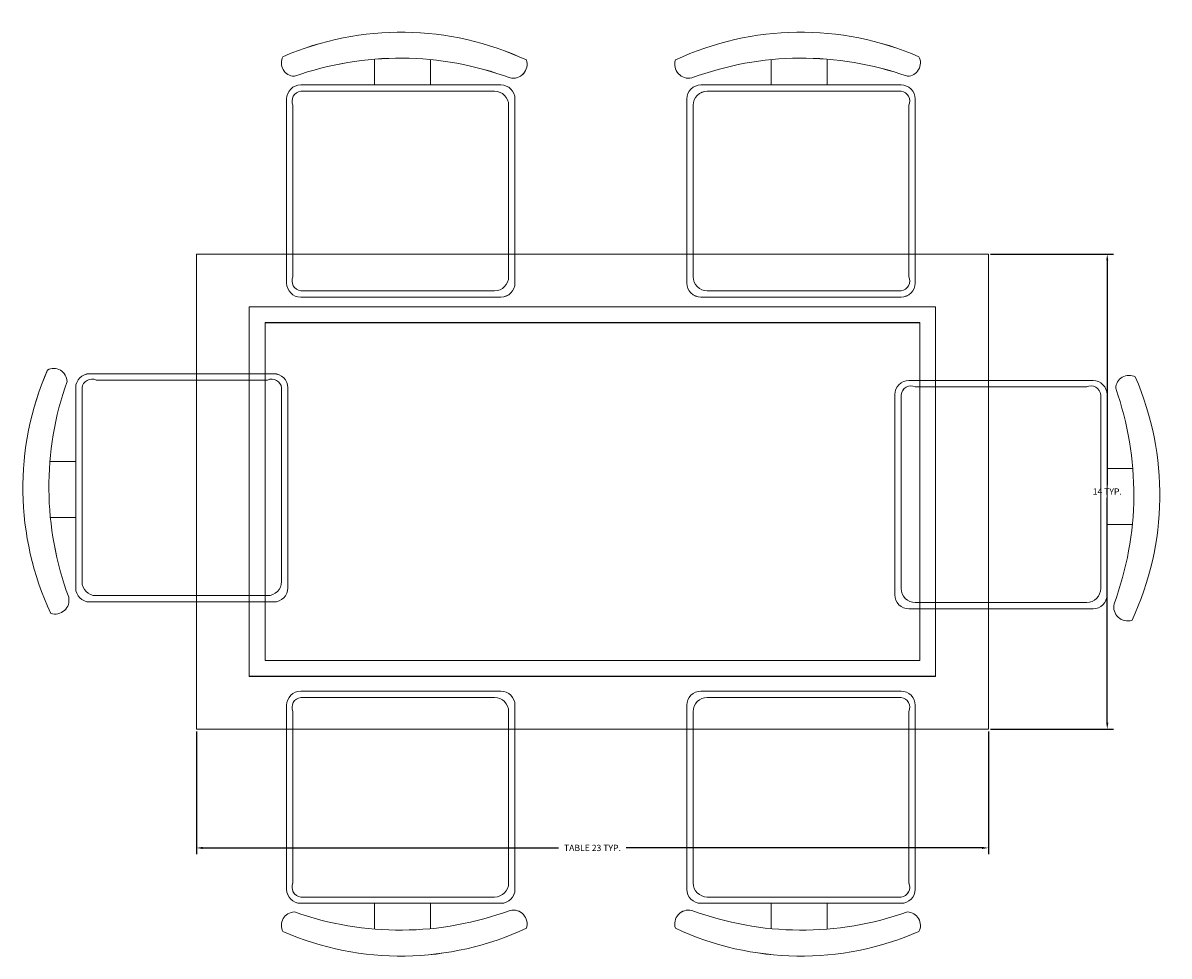
# Model space of a CAD drawing. Units: inches. Extents: x 1962 to 2771, y 1245 to 2660.
# Tile 6 of 114: x 2249 to 2281, y 1755 to 1781. Entities that reach past the tile are written whole.
import ezdxf

# ---------------------------------------------------------------- set-up
doc = ezdxf.new("R2010")
doc.units = ezdxf.units.IN
doc.layers.add('A-ANNO-DIMS', color=2, linetype='Continuous', lineweight=18)
doc.layers.add('A-FURN', color=8, linetype='Continuous', lineweight=13)
doc.styles.get("Standard").update_dxf_attribs({"font": 'arial.ttf'})
doc.dimstyles.get("Standard").update_dxf_attribs({"dimtxt": 0.18, "dimasz": 0.18, "dimexe": 0.18, "dimexo": 0.0625, "dimgap": 0.09, "dimtad": 0, "dimtih": 1, "dimtoh": 1, "dimdec": 4, "dimzin": 0, "dimdsep": 46, "dimtxsty": 'Standard', "dimcen": 0.09, "dimadec": 0, "dimazin": 0, "dimtfac": 1, "dimtdec": 4, "dimtofl": 0, "dimtmove": 0, "dimatfit": 3, "dimfxl": 1, "dimtolj": 1, "dimtzin": 0, "dimarcsym": 0})

# ---------------------------------------------------------------- blocks, each defined once
blk = doc.blocks.new('DINING-TABLE')
for points in [[(0, 13.512), (22.52, 13.512), (22.52, 0), (0, 0)], [(0, 13.512), (22.52, 13.512), (22.52, 0), (0, 0)], [(1.501, 12.011), (21.019, 12.011), (21.019, 1.502), (1.501, 1.502)], [(1.501, 12.011), (21.019, 12.011), (21.019, 1.501), (1.501, 1.501)], [(1.952, 11.561), (20.568, 11.561), (20.568, 1.952), (1.952, 1.952)], [(1.952, 11.56), (20.568, 11.56), (20.568, 1.952), (1.952, 1.952)]]:
    blk.add_lwpolyline(points, close=True)
blk = doc.blocks.new('DINING-CHAIR-A')
for points in [[(0.368, 6.279, -0.175809), (6.502, 6.233, 0.578392), (6.967, 6.744, 0.214524), (0.043, 6.837, 0.552014), (0.368, 6.279, -0.065079)], [(0.368, 6.279, -0.175809), (6.502, 6.232, 0.578392), (6.967, 6.743, 0.214524), (0.043, 6.836, 0.552014), (0.368, 6.279, -0.065079)], [(4.242, 6.033), (4.242, 6.753, -0.064759)], [(4.242, 6.033), (4.242, 6.753, -0.064759)], [(6.242, 6.033), (0.548, 6.033, 0.414214), (0.149, 5.635), (0.149, 0.399, 0.414214), (0.548, 0), (6.242, 0, 0.414214), (6.64, 0.399), (6.64, 5.635, 0.414214), (6.242, 6.033)], [(6.242, 6.033), (0.548, 6.033, 0.414214), (0.149, 5.634), (0.149, 0.398, 0.414214), (0.548, 0), (6.242, 0, 0.414214), (6.641, 0.398), (6.641, 5.634, 0.414214), (6.242, 6.033)]]:
    blk.add_lwpolyline(points, format="xyb")
blk.add_lwpolyline([(2.648, 6.766), (2.648, 6.033)])
blk.add_lwpolyline([(2.648, 6.766), (2.648, 6.033)])
for points in [[(0.55, 5.853), (6.063, 5.853, -0.414214), (6.461, 5.455), (6.461, 0.578, -0.414214), (6.063, 0.18), (0.55, 0.18, -0.512069), (0.329, 0.578), (0.329, 5.455, -0.512069)], [(0.55, 5.853), (6.063, 5.853, -0.414214), (6.461, 5.455), (6.461, 0.578, -0.414214), (6.063, 0.179), (0.55, 0.179, -0.512069), (0.329, 0.578), (0.329, 5.455, -0.512069)]]:
    blk.add_lwpolyline(points, format="xyb", close=True)
blk = doc.blocks.new('DINING-CHAIR-B')
for points in [[(6.279, 6.618, -0.175809), (6.232, 0.484, 0.578392), (6.743, 0.019, 0.214524), (6.836, 6.943, 0.552014), (6.279, 6.618, -0.065079)], [(6.279, 6.618, -0.175809), (6.232, 0.484, 0.578392), (6.743, 0.019, 0.214524), (6.836, 6.943, 0.552014), (6.279, 6.618, -0.065079)], [(6.033, 6.439, 0.414214), (5.634, 6.837), (0.398, 6.837, 0.414214), (0, 6.439), (0, 0.744, 0.414214), (0.398, 0.346), (5.634, 0.346, 0.414214), (6.033, 0.744), (6.033, 6.439)], [(6.033, 6.438, 0.414214), (5.634, 6.837), (0.398, 6.837, 0.414214), (0, 6.438), (0, 0.744, 0.414214), (0.398, 0.346), (5.634, 0.346, 0.414214), (6.033, 0.744), (6.033, 6.438)], [(6.033, 2.744), (6.753, 2.744, -0.064759)], [(6.033, 2.744), (6.753, 2.744, -0.064759)]]:
    blk.add_lwpolyline(points, format="xyb")
for points in [[(5.853, 6.436), (5.853, 0.924, -0.414214), (5.455, 0.525), (0.578, 0.525, -0.414214), (0.179, 0.924), (0.179, 6.436, -0.512069), (0.578, 6.658), (5.455, 6.658, -0.512069)], [(5.853, 6.436), (5.853, 0.923, -0.414214), (5.455, 0.525), (0.578, 0.525, -0.414214), (0.179, 0.923), (0.179, 6.436, -0.512069), (0.578, 6.657), (5.455, 6.657, -0.512069)]]:
    blk.add_lwpolyline(points, format="xyb", close=True)
blk.add_lwpolyline([(6.766, 4.338), (6.033, 4.338)])
blk.add_lwpolyline([(6.766, 4.338), (6.033, 4.338)])
blk = doc.blocks.new('*D32')
at = {"layer": 'A-ANNO-DIMS', "color": 0, "lineweight": -2, "transparency": 16777216}
for p, q in [((2253.775, 1761.339), (2253.775, 1757.843)), ((2276.295, 1761.339), (2276.295, 1757.843)), ((2253.955, 1758.023), (2264.071, 1758.023)), ((2276.115, 1758.023), (2265.998, 1758.023))]:
    blk.add_line(p, q, dxfattribs=at)
at = {"layer": 'A-ANNO-DIMS', "color": 0, "transparency": 16777216}
for points in [[(2253.955, 1758.053), (2253.955, 1757.993), (2253.775, 1758.023)], [(2276.115, 1758.053), (2276.115, 1757.993), (2276.295, 1758.023)]]:
    blk.add_solid(points, dxfattribs=at)
at = {"layer": 'Defpoints', "color": 0, "transparency": 16777216}
for p in [(2253.775, 1761.402), (2276.295, 1761.402), (2276.295, 1758.023)]:
    blk.add_point(p, dxfattribs=at)
at = {"layer": 'A-ANNO-DIMS', "color": 0, "transparency": 16777216, "insert": (2265.035, 1758.023), "char_height": 0.18, "attachment_point": 5}
blk.add_mtext('\\A1;TABLE 23 TYP.', dxfattribs=at)
blk = doc.blocks.new('*D33')
at = {"layer": 'A-ANNO-DIMS', "color": 0, "lineweight": -2, "transparency": 16777216}
for p, q in [((2276.357, 1774.914), (2279.853, 1774.914)), ((2279.673, 1774.734), (2279.673, 1768.338)), ((2279.673, 1761.582), (2279.673, 1767.977)), ((2276.357, 1761.402), (2279.853, 1761.402))]:
    blk.add_line(p, q, dxfattribs=at)
at = {"layer": 'A-ANNO-DIMS', "color": 0, "transparency": 16777216}
for points in [[(2279.643, 1774.734), (2279.703, 1774.734), (2279.673, 1774.914)], [(2279.643, 1761.582), (2279.703, 1761.582), (2279.673, 1761.402)]]:
    blk.add_solid(points, dxfattribs=at)
at = {"layer": 'Defpoints', "color": 0, "transparency": 16777216}
for p in [(2276.295, 1774.914), (2279.673, 1774.914), (2276.295, 1761.402)]:
    blk.add_point(p, dxfattribs=at)
at = {"layer": 'A-ANNO-DIMS', "color": 0, "transparency": 16777216, "insert": (2279.673, 1768.158), "char_height": 0.18, "attachment_point": 5}
blk.add_mtext('\\A1;14 TYP.', dxfattribs=at)

msp = doc.modelspace()

# ---------------------------------------------------------------- linework, layer by layer
at = {"layer": 'A-FURN'}
for points in [[(2267.8581, 1779.9227, -0.5783921), (2267.3934, 1780.4337, -0.2145244), (2274.3172, 1780.5266, -0.552014), (2273.9919, 1779.9692, 0.1758092), (2267.8581, 1779.9227)], [(2267.8581, 1779.9225, -0.5783921), (2267.3934, 1780.4334, -0.2145244), (2274.3172, 1780.5263, -0.552014), (2273.9919, 1779.9689, 0.1758092), (2267.8581, 1779.9225)], [(2270.1185, 1779.723), (2270.1185, 1780.4432, 0.0647586)], [(2270.1185, 1779.7228), (2270.1185, 1780.4429, 0.0647586)], [(2273.8128, 1779.723, -0.4142136), (2274.2112, 1779.3246), (2274.2112, 1774.0886, -0.4142136), (2273.8128, 1773.6903), (2268.1183, 1773.6903, -0.4142136), (2267.7199, 1774.0886), (2267.7199, 1779.3246, -0.4142136), (2268.1183, 1779.723), (2273.8128, 1779.723)], [(2273.8128, 1779.7228, -0.4142136), (2274.2112, 1779.3244), (2274.2112, 1774.0884, -0.4142136), (2273.8128, 1773.69), (2268.1183, 1773.69, -0.4142136), (2267.7199, 1774.0884), (2267.7199, 1779.3244, -0.4142136), (2268.1183, 1779.7228), (2273.8128, 1779.7228)], [(2250.1431, 1765.1568, -0.5783921), (2249.6321, 1764.6921, -0.2145244), (2249.5392, 1771.616, -0.552014), (2250.0966, 1771.2907, 0.1758094), (2250.1431, 1765.1568)], [(2250.1431, 1765.1566, -0.5783921), (2249.6321, 1764.6919, -0.2145244), (2249.5392, 1771.6157, -0.552014), (2250.0966, 1771.2905, 0.1758094), (2250.1431, 1765.1566)], [(2250.3428, 1771.1115, -0.4142136), (2250.7412, 1771.5099), (2255.9772, 1771.5099, -0.4142136), (2256.3756, 1771.1115), (2256.3756, 1765.4171, -0.4142136), (2255.9772, 1765.0187), (2250.7412, 1765.0187, -0.4142136), (2250.3428, 1765.4171), (2250.3428, 1771.1115)], [(2250.3428, 1771.1113, -0.4142136), (2250.7412, 1771.5097), (2255.9772, 1771.5097, -0.4142136), (2256.3756, 1771.1113), (2256.3756, 1765.4168, -0.4142136), (2255.9772, 1765.0184), (2250.7412, 1765.0184, -0.4142136), (2250.3428, 1765.4168), (2250.3428, 1771.1113)], [(2250.3428, 1767.4172), (2249.6226, 1767.4172, 0.0647586)], [(2250.3428, 1767.417), (2249.6227, 1767.417, 0.0647586)], [(2262.4339, 1756.4479), (2256.7394, 1756.4479, -0.4142136), (2256.341, 1756.8463), (2256.341, 1762.0822, -0.4142136), (2256.7394, 1762.4806), (2262.4339, 1762.4806, -0.4142136), (2262.8323, 1762.0822), (2262.8323, 1756.8463, -0.4142136), (2262.4339, 1756.4479)], [(2262.4339, 1756.4477), (2256.7394, 1756.4477, -0.4142136), (2256.3411, 1756.846), (2256.3411, 1762.082, -0.4142136), (2256.7394, 1762.4804), (2262.4339, 1762.4804, -0.4142136), (2262.8323, 1762.082), (2262.8323, 1756.846, -0.4142136), (2262.4339, 1756.4477)], [(2273.8128, 1756.4479, 0.4142136), (2274.2112, 1756.8463), (2274.2112, 1762.0822, 0.4142136), (2273.8128, 1762.4806), (2268.1183, 1762.4806, 0.4142136), (2267.7199, 1762.0822), (2267.7199, 1756.8463, 0.4142136), (2268.1183, 1756.4479), (2273.8128, 1756.4479)], [(2273.8128, 1756.4477, 0.4142136), (2274.2112, 1756.846), (2274.2112, 1762.082, 0.4142136), (2273.8128, 1762.4804), (2268.1183, 1762.4804, 0.4142136), (2267.7199, 1762.082), (2267.7199, 1756.846, 0.4142136), (2268.1183, 1756.4477), (2273.8128, 1756.4477)], [(2262.6941, 1756.2482, -0.5783921), (2263.1588, 1755.7372, -0.2145244), (2256.235, 1755.6443, -0.552014), (2256.5603, 1756.2017, 0.1758093), (2262.6941, 1756.2482)], [(2262.6942, 1756.2479, -0.5783921), (2263.1588, 1755.737, -0.2145244), (2256.235, 1755.6441, -0.552014), (2256.5603, 1756.2015, 0.1758093), (2262.6942, 1756.2479)], [(2260.4337, 1756.4479), (2260.4337, 1755.7277, 0.0647586)], [(2260.4337, 1756.4477), (2260.4337, 1755.7275, 0.0647586)], [(2273.9919, 1756.2017, -0.1758093), (2267.8581, 1756.2482, 0.5783921), (2267.3934, 1755.7372, 0.2145244), (2274.3172, 1755.6443, 0.552014), (2273.9919, 1756.2017, -0.065079)], [(2273.9919, 1756.2015, -0.1758093), (2267.8581, 1756.2479, 0.5783921), (2267.3934, 1755.737, 0.2145244), (2274.3172, 1755.6441, 0.552014), (2273.9919, 1756.2015, -0.065079)], [(2270.1185, 1756.4479), (2270.1185, 1755.7277, -0.0647586)], [(2270.1185, 1756.4477), (2270.1185, 1755.7275, -0.0647586)]]:
    msp.add_lwpolyline(points, format="xyb", dxfattribs=at)
for points in [[(2271.7124, 1780.4563), (2271.7124, 1779.723)], [(2271.7125, 1780.456), (2271.7125, 1779.7228)], [(2249.6096, 1769.0112), (2250.3428, 1769.0112)], [(2249.6096, 1769.011), (2250.3428, 1769.011)], [(2258.8398, 1755.7146), (2258.8398, 1756.4479)], [(2258.8398, 1755.7144), (2258.8398, 1756.4477)], [(2271.7124, 1755.7146), (2271.7124, 1756.4479)], [(2271.7125, 1755.7144), (2271.7125, 1756.4477)]]:
    msp.add_lwpolyline(points, dxfattribs=at)
for points in [[(2273.8103, 1779.5435), (2268.2978, 1779.5435, 0.4142136), (2267.8994, 1779.1451), (2267.8994, 1774.2681, 0.4142136), (2268.2978, 1773.8697), (2273.8103, 1773.8697, 0.5120695), (2274.0317, 1774.2681), (2274.0317, 1779.1451, 0.5120695)], [(2273.8104, 1779.5433), (2268.2978, 1779.5433, 0.4142136), (2267.8994, 1779.1449), (2267.8994, 1774.2679, 0.4142136), (2268.2978, 1773.8695), (2273.8104, 1773.8695, 0.5120695), (2274.0317, 1774.2679), (2274.0317, 1779.1449, 0.5120695)], [(2250.5223, 1771.1091), (2250.5223, 1765.5965, 0.4142136), (2250.9207, 1765.1981), (2255.7977, 1765.1981, 0.4142136), (2256.1961, 1765.5965), (2256.1961, 1771.1091, 0.5120695), (2255.7977, 1771.3304), (2250.9207, 1771.3304, 0.5120695)], [(2250.5223, 1771.1089), (2250.5223, 1765.5963, 0.4142136), (2250.9207, 1765.1979), (2255.7977, 1765.1979, 0.4142136), (2256.1961, 1765.5963), (2256.1961, 1771.1089, 0.5120695), (2255.7977, 1771.3302), (2250.9207, 1771.3302, 0.5120695)], [(2256.7419, 1756.6274), (2262.2544, 1756.6274, 0.4142136), (2262.6528, 1757.0258), (2262.6528, 1761.9028, 0.4142136), (2262.2544, 1762.3011), (2256.7419, 1762.3011, 0.5120695), (2256.5205, 1761.9028), (2256.5205, 1757.0258, 0.5120695)], [(2256.7419, 1756.6271), (2262.2544, 1756.6271, 0.4142136), (2262.6528, 1757.0255), (2262.6528, 1761.9025, 0.4142136), (2262.2544, 1762.3009), (2256.7419, 1762.3009, 0.5120695), (2256.5205, 1761.9025), (2256.5205, 1757.0255, 0.5120695)], [(2273.8103, 1756.6274), (2268.2978, 1756.6274, -0.4142136), (2267.8994, 1757.0258), (2267.8994, 1761.9028, -0.4142136), (2268.2978, 1762.3011), (2273.8103, 1762.3011, -0.5120695), (2274.0317, 1761.9028), (2274.0317, 1757.0258, -0.5120695)], [(2273.8104, 1756.6271), (2268.2978, 1756.6271, -0.4142136), (2267.8994, 1757.0255), (2267.8994, 1761.9025, -0.4142136), (2268.2978, 1762.3009), (2273.8104, 1762.3009, -0.5120695), (2274.0317, 1761.9025), (2274.0317, 1757.0255, -0.5120695)]]:
    msp.add_lwpolyline(points, format="xyb", close=True, dxfattribs=at)

# ---------------------------------------------------------------- block references
for name, p in [('DINING-CHAIR-A', (2256.1918, 1773.69)), ('DINING-TABLE', (2253.7748, 1761.4015)), ('DINING-CHAIR-B', (2273.6339, 1764.4778))]:
    msp.add_blockref(name, p, dxfattribs=at)

# ---------------------------------------------------------------- dimensions: what is measured, and where the dimension line sits
at = {"layer": 'A-ANNO-DIMS'}
dim = msp.add_linear_dim(base=(2279.673, 1774.9139), p1=(2276.295, 1761.4015), p2=(2276.295, 1774.9139), angle=90, text='<> TYP.', dimstyle='Standard', override={"dimdec": 0, "dimlfac": 1, "dimrnd": 0, "dimzin": 0, "dimdsep": 46, "dimlunit": 2}, dxfattribs=at)
dim.commit()
dim.dimension.update_dxf_attribs({"geometry": '*D33', "text_midpoint": (2279.673, 1768.1577)})
dim = msp.add_linear_dim(base=(2276.295, 1758.0235), p1=(2253.7748, 1761.4015), p2=(2276.295, 1761.4015), text='TABLE <> TYP.', dimstyle='Standard', override={"dimdec": 0, "dimlfac": 1, "dimrnd": 0, "dimzin": 0, "dimdsep": 46, "dimlunit": 2}, dxfattribs=at)
dim.commit()
dim.dimension.update_dxf_attribs({"geometry": '*D32', "text_midpoint": (2265.0349, 1758.0235)})

doc.saveas('drawing.dxf')
